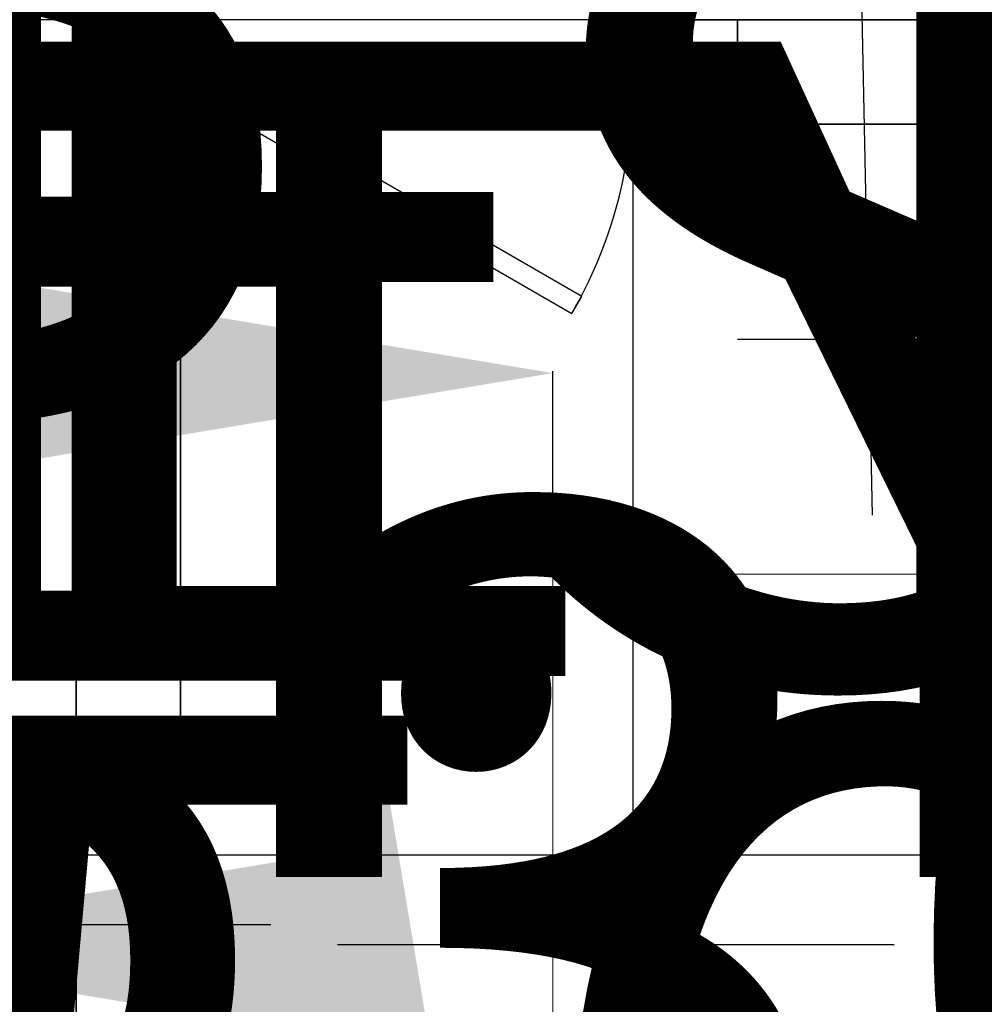
# Model space of a CAD drawing. Units: inches. Extents: x -307 to 2141, y -58 to 895.
# Tile 15 of 28: x 749 to 833, y 396 to 481. Entities that reach past the tile are written whole.
import ezdxf

# ---------------------------------------------------------------- set-up
doc = ezdxf.new("R2010")
doc.units = ezdxf.units.IN
doc.header["$MEASUREMENT"] = 0
for name, color, linetype, lineweight in [('A-ANNO-DIMS', 2, 'Continuous', 18), ('A-DOOR', 3, 'Continuous', 25), ('A-FURN', 8, 'Continuous', 18), ('A-WALL', 7, 'Continuous', 35)]:
    doc.layers.add(name, color=color, linetype=linetype, lineweight=lineweight)
doc.styles.get("Standard").update_dxf_attribs({"font": 'arial.ttf'})
doc.dimstyles.get("Standard").update_dxf_attribs({"dimtxt": 72, "dimasz": 48, "dimexe": 0.18, "dimexo": 0.0625, "dimgap": 0.09, "dimtad": 0, "dimtih": 1, "dimtoh": 1, "dimdec": 0, "dimrnd": 48, "dimzin": 0, "dimdsep": 46, "dimlunit": 3, "dimtxsty": 'Standard', "dimcen": 0.09, "dimadec": 0, "dimazin": 0, "dimtfac": 1, "dimtdec": 0, "dimtofl": 0, "dimtmove": 0, "dimatfit": 3, "dimfxl": 1, "dimtolj": 1, "dimtzin": 0, "dimarcsym": 0})

# ---------------------------------------------------------------- blocks, each defined once
blk = doc.blocks.new('*U5')
for p, q in [((0, 0), (0, -6)), ((-40, 0), (-40, -6))]:
    blk.add_line(p, q)
blk.add_lwpolyline([(0, 0), (-34.641, 20), (-35.516, 18.484), (-0.875, -1.516)], close=True)
blk.add_arc((0, 0), 40, 150, 180)
blk = doc.blocks.new('Bed - Queen')
for p, q in [((59.99999, 0), (59.99999, -80.00003)), ((59.99999, -80.00003), (0, -80.00003))]:
    blk.add_line(p, q)
blk = doc.blocks.new('*D28')
at = {"layer": 'A-ANNO-DIMS', "color": 0, "lineweight": -2, "transparency": 16777216}
for p, q in [((795.358, 433.55), (777.919, 433.55)), ((778.099, 385.55), (778.099, 366.073)), ((795.358, 318.073), (777.919, 318.073)), ((778.099, 318.073), (778.099, 270.073)), ((778.099, 270.073), (730.099, 270.073))]:
    blk.add_line(p, q, dxfattribs=at)
at = {"layer": 'A-ANNO-DIMS', "color": 0, "transparency": 16777216}
for points in [[(770.099, 385.55), (786.099, 385.55), (778.099, 433.55)], [(770.099, 366.073), (786.099, 366.073), (778.099, 318.073)]]:
    blk.add_solid(points, dxfattribs=at)
at = {"layer": 'Defpoints', "color": 0, "transparency": 16777216}
for p in [(795.421, 433.55), (778.099, 318.073), (795.421, 318.073)]:
    blk.add_point(p, dxfattribs=at)
at = {"layer": 'A-ANNO-DIMS', "color": 0, "transparency": 16777216, "insert": (534.416, 270.073), "char_height": 72, "attachment_point": 5}
blk.add_mtext('\\A1;BED 115', dxfattribs=at)
blk = doc.blocks.new('*D29')
at = {"layer": 'A-ANNO-DIMS', "color": 0, "lineweight": -2, "transparency": 16777216}
for p, q in [((747.421, 450.871), (699.421, 450.871)), ((795.421, 433.612), (795.421, 451.051)), ((882.028, 433.612), (882.028, 451.051)), ((930.028, 450.871), (978.028, 450.871))]:
    blk.add_line(p, q, dxfattribs=at)
at = {"layer": 'A-ANNO-DIMS', "color": 0, "transparency": 16777216}
for points in [[(747.421, 458.871), (747.421, 442.871), (795.421, 450.871)], [(930.028, 458.871), (930.028, 442.871), (882.028, 450.871)]]:
    blk.add_solid(points, dxfattribs=at)
at = {"layer": 'Defpoints', "color": 0, "transparency": 16777216}
for p in [(795.421, 450.871), (795.421, 433.55), (882.028, 433.55)]:
    blk.add_point(p, dxfattribs=at)
at = {"layer": 'A-ANNO-DIMS', "color": 0, "transparency": 16777216, "insert": (647.713, 450.871), "char_height": 72, "attachment_point": 5}
blk.add_mtext('\\A1;87', dxfattribs=at)
blk = doc.blocks.new('*D30')
at = {"layer": 'A-ANNO-DIMS', "color": 0, "lineweight": -2, "transparency": 16777216}
for p, q in [((570.736, 532.833), (570.736, 580.833)), ((570.736, 580.833), (618.736, 580.833)), ((565.398, 484.833), (570.916, 484.833)), ((565.398, 448.833), (570.916, 448.833)), ((570.736, 400.833), (570.736, 352.833))]:
    blk.add_line(p, q, dxfattribs=at)
at = {"layer": 'A-ANNO-DIMS', "color": 0, "transparency": 16777216}
for points in [[(562.736, 532.833), (578.736, 532.833), (570.736, 484.833)], [(562.736, 400.833), (578.736, 400.833), (570.736, 448.833)]]:
    blk.add_solid(points, dxfattribs=at)
at = {"layer": 'Defpoints', "color": 0, "transparency": 16777216}
for p in [(565.336, 484.833), (570.736, 484.833), (565.336, 448.833)]:
    blk.add_point(p, dxfattribs=at)
at = {"layer": 'A-ANNO-DIMS', "color": 0, "transparency": 16777216, "insert": (1030.174, 580.833), "char_height": 72, "attachment_point": 5}
blk.add_mtext('\\A1;WINDOW 36 TYP.', dxfattribs=at)
blk = doc.blocks.new('*D31')
at = {"layer": 'A-ANNO-DIMS', "color": 0, "lineweight": -2, "transparency": 16777216}
for p, q in [((556.336, 448.771), (556.336, 443.253)), ((565.336, 448.771), (565.336, 443.253)), ((508.336, 443.433), (460.336, 443.433)), ((613.336, 443.433), (661.336, 443.433))]:
    blk.add_line(p, q, dxfattribs=at)
at = {"layer": 'A-ANNO-DIMS', "color": 0, "transparency": 16777216}
for points in [[(508.336, 451.433), (508.336, 435.433), (556.336, 443.433)], [(613.336, 451.433), (613.336, 435.433), (565.336, 443.433)]]:
    blk.add_solid(points, dxfattribs=at)
at = {"layer": 'Defpoints', "color": 0, "transparency": 16777216}
for p in [(556.336, 448.833), (565.336, 448.833), (565.336, 443.433)]:
    blk.add_point(p, dxfattribs=at)
at = {"layer": 'A-ANNO-DIMS', "color": 0, "transparency": 16777216, "insert": (808.692, 443.433), "char_height": 72, "attachment_point": 5}
blk.add_mtext('\\A1;9 TYP.', dxfattribs=at)
blk = doc.blocks.new('*D35')
at = {"layer": 'A-ANNO-DIMS', "color": 0, "lineweight": -2, "transparency": 16777216}
for p, q in [((859.336, 453.769), (811.336, 453.769)), ((907.336, 443.029), (907.336, 453.949)), ((916.336, 443.029), (916.336, 453.949)), ((964.336, 453.769), (1012.336, 453.769))]:
    blk.add_line(p, q, dxfattribs=at)
at = {"layer": 'A-ANNO-DIMS', "color": 0, "transparency": 16777216}
for points in [[(859.336, 461.769), (859.336, 445.769), (907.336, 453.769)], [(964.336, 461.769), (964.336, 445.769), (916.336, 453.769)]]:
    blk.add_solid(points, dxfattribs=at)
at = {"layer": 'Defpoints', "color": 0, "transparency": 16777216}
for p in [(907.336, 453.769), (907.336, 442.967), (916.336, 442.967)]:
    blk.add_point(p, dxfattribs=at)
at = {"layer": 'A-ANNO-DIMS', "color": 0, "transparency": 16777216, "insert": (663.98, 453.769), "char_height": 72, "attachment_point": 5}
blk.add_mtext('\\A1;9 TYP.', dxfattribs=at)
blk = doc.blocks.new('*D36')
at = {"layer": 'A-ANNO-DIMS', "color": 0, "lineweight": -2, "transparency": 16777216}
for p, q in [((871.707, 562.404), (871.761, 610.404)), ((876.548, 514.399), (871.474, 514.405)), ((876.511, 481.353), (871.437, 481.358)), ((871.563, 433.358), (871.509, 385.358)), ((871.509, 385.358), (823.509, 385.358))]:
    blk.add_line(p, q, dxfattribs=at)
at = {"layer": 'A-ANNO-DIMS', "color": 0, "transparency": 16777216}
for points in [[(863.707, 562.413), (879.707, 562.395), (871.654, 514.404)], [(863.563, 433.367), (879.563, 433.349), (871.617, 481.358)]]:
    blk.add_solid(points, dxfattribs=at)
at = {"layer": 'Defpoints', "color": 0, "transparency": 16777216}
for p in [(876.611, 514.399), (871.617, 481.358), (876.574, 481.353)]:
    blk.add_point(p, dxfattribs=at)
at = {"layer": 'A-ANNO-DIMS', "color": 0, "transparency": 16777216, "insert": (548.95, 385.358), "char_height": 72, "attachment_point": 5}
blk.add_mtext('\\A1;WC 33 TYP.', dxfattribs=at)
blk = doc.blocks.new('*D37')
at = {"layer": 'A-ANNO-DIMS', "color": 0, "lineweight": -2, "transparency": 16777216}
for p, q in [((876.611, 514.461), (876.616, 519.536)), ((828.616, 519.409), (780.616, 519.463)), ((897.611, 514.438), (897.616, 519.512)), ((945.616, 519.279), (993.616, 519.225))]:
    blk.add_line(p, q, dxfattribs=at)
at = {"layer": 'A-ANNO-DIMS', "color": 0, "transparency": 16777216}
for points in [[(828.625, 527.409), (828.607, 511.409), (876.616, 519.356)], [(945.625, 527.279), (945.607, 511.279), (897.616, 519.332)]]:
    blk.add_solid(points, dxfattribs=at)
at = {"layer": 'Defpoints', "color": 0, "transparency": 16777216}
for p in [(876.616, 519.356), (876.611, 514.399), (897.611, 514.375)]:
    blk.add_point(p, dxfattribs=at)
at = {"layer": 'A-ANNO-DIMS', "color": 0, "transparency": 16777216, "insert": (604.676, 519.463), "char_height": 72, "attachment_point": 5}
blk.add_mtext('\\A1;21 TYP.', dxfattribs=at)
blk = doc.blocks.new('*D42')
at = {"layer": 'A-ANNO-DIMS', "color": 0, "lineweight": -2, "transparency": 16777216}
for p, q in [((880.259, 543.859), (928.248, 544.868)), ((822.302, 541.203), (822.268, 542.82)), ((832.299, 541.413), (832.265, 543.03)), ((774.282, 541.631), (726.293, 540.622))]:
    blk.add_line(p, q, dxfattribs=at)
at = {"layer": 'A-ANNO-DIMS', "color": 0, "transparency": 16777216}
for points in [[(880.09, 551.857), (880.427, 535.861), (832.269, 542.85)], [(774.114, 549.629), (774.45, 533.633), (822.271, 542.64)]]:
    blk.add_solid(points, dxfattribs=at)
at = {"layer": 'Defpoints', "color": 0, "transparency": 16777216}
for p in [(832.269, 542.85), (822.303, 541.14), (832.301, 541.35)]:
    blk.add_point(p, dxfattribs=at)
at = {"layer": 'A-ANNO-DIMS', "color": 0, "transparency": 16777216, "insert": (1192.886, 544.868), "char_height": 72, "attachment_point": 5}
blk.add_mtext('\\A1;FAUCET 10', dxfattribs=at)
blk = doc.blocks.new('*D43')
at = {"layer": 'A-ANNO-DIMS', "color": 0, "lineweight": -2, "transparency": 16777216}
for p, q in [((818.785, 637.088), (770.785, 637.088)), ((819.794, 589.098), (818.785, 637.088)), ((822.24, 541.139), (820.623, 541.105)), ((822.377, 534.64), (820.76, 534.606)), ((821.949, 486.621), (822.958, 438.631))]:
    blk.add_line(p, q, dxfattribs=at)
at = {"layer": 'A-ANNO-DIMS', "color": 0, "transparency": 16777216}
for points in [[(827.792, 589.266), (811.796, 588.93), (820.803, 541.109)], [(829.947, 486.789), (813.951, 486.453), (820.94, 534.61)]]:
    blk.add_solid(points, dxfattribs=at)
at = {"layer": 'Defpoints', "color": 0, "transparency": 16777216}
for p in [(820.803, 541.109), (822.303, 541.14), (822.44, 534.642)]:
    blk.add_point(p, dxfattribs=at)
at = {"layer": 'A-ANNO-DIMS', "color": 0, "transparency": 16777216, "insert": (747.391, 637.088), "char_height": 72, "attachment_point": 5}
blk.add_mtext('\\A1;7', dxfattribs=at)
blk = doc.blocks.new('*D44')
at = {"layer": 'A-ANNO-DIMS', "color": 0, "lineweight": -2, "transparency": 16777216}
for p, q in [((839.872, 521.223), (839.952, 517.424)), ((815.327, 520.707), (815.406, 516.907)), ((887.938, 518.613), (935.927, 519.622)), ((767.413, 516.078), (719.424, 515.069))]:
    blk.add_line(p, q, dxfattribs=at)
at = {"layer": 'A-ANNO-DIMS', "color": 0, "transparency": 16777216}
for points in [[(887.769, 526.611), (888.106, 510.614), (839.948, 517.604)], [(767.245, 524.076), (767.581, 508.08), (815.403, 517.087)]]:
    blk.add_solid(points, dxfattribs=at)
at = {"layer": 'Defpoints', "color": 0, "transparency": 16777216}
for p in [(839.871, 521.285), (815.325, 520.769), (839.948, 517.604)]:
    blk.add_point(p, dxfattribs=at)
at = {"layer": 'A-ANNO-DIMS', "color": 0, "transparency": 16777216, "insert": (1151.157, 519.622), "char_height": 72, "attachment_point": 5}
blk.add_mtext('\\A1;BASIN 25', dxfattribs=at)
blk = doc.blocks.new('*D45')
at = {"layer": 'A-ANNO-DIMS', "color": 0, "lineweight": -2, "transparency": 16777216}
for p, q in [((841.111, 637.474), (793.111, 637.474)), ((842.12, 589.484), (841.111, 637.474)), ((839.51, 541.419), (843.309, 541.499)), ((839.933, 521.287), (843.732, 521.367)), ((844.562, 473.373), (845.571, 425.384))]:
    blk.add_line(p, q, dxfattribs=at)
at = {"layer": 'A-ANNO-DIMS', "color": 0, "transparency": 16777216}
for points in [[(850.118, 589.652), (834.122, 589.316), (843.129, 541.495)], [(852.56, 473.542), (836.563, 473.205), (843.553, 521.363)]]:
    blk.add_solid(points, dxfattribs=at)
at = {"layer": 'Defpoints', "color": 0, "transparency": 16777216}
for p in [(839.447, 541.417), (843.129, 541.495), (839.871, 521.285)]:
    blk.add_point(p, dxfattribs=at)
at = {"layer": 'A-ANNO-DIMS', "color": 0, "transparency": 16777216, "insert": (740.961, 637.474), "char_height": 72, "attachment_point": 5}
blk.add_mtext('\\A1;20', dxfattribs=at)
blk = doc.blocks.new('*D46')
at = {"layer": 'A-ANNO-DIMS', "color": 0, "lineweight": -2, "transparency": 16777216}
for p, q in [((801.413, 645.783), (801.413, 642.516)), ((822.413, 645.783), (822.413, 642.516)), ((753.413, 642.696), (705.413, 642.696)), ((870.413, 642.696), (918.413, 642.696))]:
    blk.add_line(p, q, dxfattribs=at)
at = {"layer": 'A-ANNO-DIMS', "color": 0, "transparency": 16777216}
for points in [[(753.413, 650.696), (753.413, 634.696), (801.413, 642.696)], [(870.413, 650.696), (870.413, 634.696), (822.413, 642.696)]]:
    blk.add_solid(points, dxfattribs=at)
at = {"layer": 'Defpoints', "color": 0, "transparency": 16777216}
for p in [(801.413, 645.846), (822.413, 645.846), (822.413, 642.696)]:
    blk.add_point(p, dxfattribs=at)
at = {"layer": 'A-ANNO-DIMS', "color": 0, "transparency": 16777216, "insert": (1282.702, 642.696), "char_height": 72, "attachment_point": 5}
blk.add_mtext('\\A1;DESK CHAIR 21', dxfattribs=at)
blk = doc.blocks.new('*D52')
at = {"layer": 'A-ANNO-DIMS', "color": 0, "lineweight": -2, "transparency": 16777216}
for p, q in [((660.208, 554.249), (660.208, 602.249)), ((673.796, 506.249), (660.028, 506.249)), ((673.796, 415.249), (660.028, 415.249)), ((660.208, 367.249), (660.208, 319.249))]:
    blk.add_line(p, q, dxfattribs=at)
at = {"layer": 'A-ANNO-DIMS', "color": 0, "transparency": 16777216}
for points in [[(652.208, 554.249), (668.208, 554.249), (660.208, 506.249)], [(652.208, 367.249), (668.208, 367.249), (660.208, 415.249)]]:
    blk.add_solid(points, dxfattribs=at)
at = {"layer": 'Defpoints', "color": 0, "transparency": 16777216}
for p in [(673.858, 506.249), (660.208, 415.249), (673.858, 415.249)]:
    blk.add_point(p, dxfattribs=at)
at = {"layer": 'A-ANNO-DIMS', "color": 0, "transparency": 16777216, "insert": (660.208, 460.749), "char_height": 72, "attachment_point": 5}
blk.add_mtext('\\A1;DINING SET 91', dxfattribs=at)
blk = doc.blocks.new('*D53')
at = {"layer": 'A-ANNO-DIMS', "color": 0, "lineweight": -2, "transparency": 16777216}
for p, q in [((673.858, 415.186), (673.858, 401.419)), ((728.858, 415.186), (728.858, 401.419)), ((625.858, 401.599), (577.858, 401.599)), ((776.858, 401.599), (824.858, 401.599))]:
    blk.add_line(p, q, dxfattribs=at)
at = {"layer": 'A-ANNO-DIMS', "color": 0, "transparency": 16777216}
for points in [[(625.858, 409.599), (625.858, 393.599), (673.858, 401.599)], [(776.858, 409.599), (776.858, 393.599), (728.858, 401.599)]]:
    blk.add_solid(points, dxfattribs=at)
at = {"layer": 'Defpoints', "color": 0, "transparency": 16777216}
for p in [(673.858, 415.249), (728.858, 415.249), (728.858, 401.599)]:
    blk.add_point(p, dxfattribs=at)
at = {"layer": 'A-ANNO-DIMS', "color": 0, "transparency": 16777216, "insert": (876.787, 401.599), "char_height": 72, "attachment_point": 5}
blk.add_mtext('\\A1;55', dxfattribs=at)
blk = doc.blocks.new('*D54')
at = {"layer": 'A-ANNO-DIMS', "color": 0, "lineweight": -2, "transparency": 16777216}
for p, q in [((605.336, 412.349), (605.336, 460.349)), ((605.336, 460.349), (653.336, 460.349)), ((596.398, 364.349), (605.516, 364.349)), ((596.398, 304.349), (605.516, 304.349)), ((605.336, 256.349), (605.336, 208.349))]:
    blk.add_line(p, q, dxfattribs=at)
at = {"layer": 'A-ANNO-DIMS', "color": 0, "transparency": 16777216}
for points in [[(597.336, 412.349), (613.336, 412.349), (605.336, 364.349)], [(597.336, 256.349), (613.336, 256.349), (605.336, 304.349)]]:
    blk.add_solid(points, dxfattribs=at)
at = {"layer": 'Defpoints', "color": 0, "transparency": 16777216}
for p in [(596.336, 364.349), (605.336, 364.349), (596.336, 304.349)]:
    blk.add_point(p, dxfattribs=at)
at = {"layer": 'A-ANNO-DIMS', "color": 0, "transparency": 16777216, "insert": (854.004, 460.349), "char_height": 72, "attachment_point": 5}
blk.add_mtext('\\A1;DESK 60', dxfattribs=at)
blk = doc.blocks.new('*D60')
at = {"layer": 'A-ANNO-DIMS', "color": 0, "lineweight": -2, "transparency": 16777216}
for p, q in [((659.857, 294.946), (659.857, 342.946)), ((659.857, 342.946), (707.857, 342.946)), ((663.339, 246.946), (659.677, 246.946)), ((663.339, 223.315), (659.677, 223.315)), ((659.857, 175.315), (659.857, 127.315))]:
    blk.add_line(p, q, dxfattribs=at)
at = {"layer": 'A-ANNO-DIMS', "color": 0, "transparency": 16777216}
for points in [[(651.857, 294.946), (667.857, 294.946), (659.857, 246.946)], [(651.857, 175.315), (667.857, 175.315), (659.857, 223.315)]]:
    blk.add_solid(points, dxfattribs=at)
at = {"layer": 'Defpoints', "color": 0, "transparency": 16777216}
for p in [(659.857, 246.946), (663.402, 246.946), (663.402, 223.315)]:
    blk.add_point(p, dxfattribs=at)
at = {"layer": 'A-ANNO-DIMS', "color": 0, "transparency": 16777216, "insert": (933.573, 342.946), "char_height": 72, "attachment_point": 5}
blk.add_mtext('\\A1;TABLE 24', dxfattribs=at)
blk = doc.blocks.new('*D63')
at = {"layer": 'A-ANNO-DIMS', "color": 0, "lineweight": -2, "transparency": 16777216}
for p, q in [((916.398, 691.341), (947.72, 691.341)), ((947.54, 643.341), (947.54, 416.192)), ((947.54, 115.341), (947.54, 342.49)), ((704.684, 67.341), (947.72, 67.341))]:
    blk.add_line(p, q, dxfattribs=at)
at = {"layer": 'A-ANNO-DIMS', "color": 0, "transparency": 16777216}
for points in [[(939.54, 643.341), (955.54, 643.341), (947.54, 691.341)], [(939.54, 115.341), (955.54, 115.341), (947.54, 67.341)]]:
    blk.add_solid(points, dxfattribs=at)
at = {"layer": 'Defpoints', "color": 0, "transparency": 16777216}
for p in [(916.336, 691.341), (704.621, 67.341), (947.54, 67.341)]:
    blk.add_point(p, dxfattribs=at)
at = {"layer": 'A-ANNO-DIMS', "color": 0, "transparency": 16777216, "insert": (947.54, 379.341), "char_height": 72, "attachment_point": 5}
blk.add_mtext('\\A1;624', dxfattribs=at)
blk = doc.blocks.new('*D68')
at = {"layer": 'A-ANNO-DIMS', "color": 0, "lineweight": -2, "transparency": 16777216}
for p, q in [((525.132, 586.341), (525.132, 634.341)), ((525.132, 634.341), (573.132, 634.341)), ((565.273, 538.341), (524.952, 538.341)), ((556.273, 484.833), (524.952, 484.833)), ((525.132, 436.833), (525.132, 388.833))]:
    blk.add_line(p, q, dxfattribs=at)
at = {"layer": 'A-ANNO-DIMS', "color": 0, "transparency": 16777216}
for points in [[(517.132, 586.341), (533.132, 586.341), (525.132, 538.341)], [(517.132, 436.833), (533.132, 436.833), (525.132, 484.833)]]:
    blk.add_solid(points, dxfattribs=at)
at = {"layer": 'Defpoints', "color": 0, "transparency": 16777216}
for p in [(525.132, 538.341), (565.336, 538.341), (556.336, 484.833)]:
    blk.add_point(p, dxfattribs=at)
at = {"layer": 'A-ANNO-DIMS', "color": 0, "transparency": 16777216, "insert": (687.754, 634.341), "char_height": 72, "attachment_point": 5}
blk.add_mtext('\\A1;53.51', dxfattribs=at)
blk = doc.blocks.new('*D82')
at = {"layer": 'A-ANNO-DIMS', "color": 0, "lineweight": -2, "transparency": 16777216}
for p, q in [((525.132, 565.341), (525.132, 613.341)), ((525.132, 613.341), (573.132, 613.341)), ((802.273, 517.341), (524.952, 517.341)), ((802.273, 481.341), (524.952, 481.341)), ((525.132, 433.341), (525.132, 385.341))]:
    blk.add_line(p, q, dxfattribs=at)
at = {"layer": 'A-ANNO-DIMS', "color": 0, "transparency": 16777216}
for points in [[(517.132, 565.341), (533.132, 565.341), (525.132, 517.341)], [(517.132, 433.341), (533.132, 433.341), (525.132, 481.341)]]:
    blk.add_solid(points, dxfattribs=at)
at = {"layer": 'Defpoints', "color": 0, "transparency": 16777216}
for p in [(525.132, 517.341), (802.336, 517.341), (802.336, 481.341)]:
    blk.add_point(p, dxfattribs=at)
at = {"layer": 'A-ANNO-DIMS', "color": 0, "transparency": 16777216, "insert": (624.742, 613.341), "char_height": 72, "attachment_point": 5}
blk.add_mtext('\\A1;36', dxfattribs=at)
blk = doc.blocks.new('*D83')
at = {"layer": 'A-ANNO-DIMS', "color": 0, "lineweight": -2, "transparency": 16777216}
for p, q in [((947.54, 538.903), (947.54, 586.903)), ((916.398, 490.903), (947.72, 490.903)), ((907.398, 481.341), (947.72, 481.341)), ((947.54, 433.341), (947.54, 385.341)), ((947.54, 385.341), (899.54, 385.341))]:
    blk.add_line(p, q, dxfattribs=at)
at = {"layer": 'A-ANNO-DIMS', "color": 0, "transparency": 16777216}
for points in [[(939.54, 538.903), (955.54, 538.903), (947.54, 490.903)], [(939.54, 433.341), (955.54, 433.341), (947.54, 481.341)]]:
    blk.add_solid(points, dxfattribs=at)
at = {"layer": 'Defpoints', "color": 0, "transparency": 16777216}
for p in [(916.336, 490.903), (907.336, 481.341), (947.54, 481.341)]:
    blk.add_point(p, dxfattribs=at)
at = {"layer": 'A-ANNO-DIMS', "color": 0, "transparency": 16777216, "insert": (777.968, 385.341), "char_height": 72, "attachment_point": 5}
blk.add_mtext('\\A1;9.563', dxfattribs=at)
blk = doc.blocks.new('*D84')
at = {"layer": 'A-ANNO-DIMS', "color": 0, "lineweight": -2, "transparency": 16777216}
for p, q in [((763.336, 472.278), (763.336, 35.957)), ((907.336, 472.278), (907.336, 35.957)), ((811.336, 36.137), (859.336, 36.137)), ((907.336, 36.137), (955.336, 36.137))]:
    blk.add_line(p, q, dxfattribs=at)
at = {"layer": 'A-ANNO-DIMS', "color": 0, "transparency": 16777216}
for points in [[(811.336, 44.137), (811.336, 28.137), (763.336, 36.137)], [(859.336, 44.137), (859.336, 28.137), (907.336, 36.137)]]:
    blk.add_solid(points, dxfattribs=at)
at = {"layer": 'Defpoints', "color": 0, "transparency": 16777216}
for p in [(763.336, 472.341), (907.336, 472.341), (907.336, 36.137)]:
    blk.add_point(p, dxfattribs=at)
at = {"layer": 'A-ANNO-DIMS', "color": 0, "transparency": 16777216, "insert": (1031.429, 36.137), "char_height": 72, "attachment_point": 5}
blk.add_mtext('\\A1;144', dxfattribs=at)
blk = doc.blocks.new('*D88')
at = {"layer": 'A-ANNO-DIMS', "color": 0, "lineweight": -2, "transparency": 16777216}
for p, q in [((517.33584, 722.544828), (469.33584, 722.544828)), ((565.33584, 295.403328), (565.33584, 722.724828)), ((754.33584, 271.403328), (754.33584, 722.724828)), ((802.33584, 722.544828), (850.33584, 722.544828))]:
    blk.add_line(p, q, dxfattribs=at)
at = {"layer": 'A-ANNO-DIMS', "color": 0, "transparency": 16777216}
for points in [[(517.33584, 730.544828), (517.33584, 714.544828), (565.33584, 722.544828)], [(802.33584, 730.544828), (802.33584, 714.544828), (754.33584, 722.544828)]]:
    blk.add_solid(points, dxfattribs=at)
at = {"layer": 'Defpoints', "color": 0, "transparency": 16777216}
for p in [(754.33584, 722.544828), (565.33584, 295.340828), (754.33584, 271.340828)]:
    blk.add_point(p, dxfattribs=at)
at = {"layer": 'A-ANNO-DIMS', "color": 0, "transparency": 16777216, "insert": (659.83584, 722.544828), "char_height": 72, "attachment_point": 5}
blk.add_mtext('\\A1;189', dxfattribs=at)
blk = doc.blocks.new('*D95')
at = {"layer": 'A-ANNO-DIMS', "color": 0, "lineweight": -2, "transparency": 16777216}
for p, q in [((947.54, 577.341), (947.54, 625.341)), ((947.54, 625.341), (995.54, 625.341)), ((629.898, 529.341), (947.72, 529.341)), ((629.898, 502.663), (947.72, 502.663)), ((947.54, 454.663), (947.54, 406.663))]:
    blk.add_line(p, q, dxfattribs=at)
at = {"layer": 'A-ANNO-DIMS', "color": 0, "transparency": 16777216}
for points in [[(939.54, 577.341), (955.54, 577.341), (947.54, 529.341)], [(939.54, 454.663), (955.54, 454.663), (947.54, 502.663)]]:
    blk.add_solid(points, dxfattribs=at)
at = {"layer": 'Defpoints', "color": 0, "transparency": 16777216}
for p in [(629.836, 529.341), (947.54, 529.341), (629.836, 502.663)]:
    blk.add_point(p, dxfattribs=at)
at = {"layer": 'A-ANNO-DIMS', "color": 0, "transparency": 16777216, "insert": (1117.799, 625.341), "char_height": 72, "attachment_point": 5}
blk.add_mtext('\\A1;26.68', dxfattribs=at)
blk = doc.blocks.new('*D97')
at = {"layer": 'A-ANNO-DIMS', "color": 0, "lineweight": -2, "transparency": 16777216}
for p, q in [((947.54, 637.341), (947.54, 685.341)), ((947.54, 685.341), (995.54, 685.341)), ((685.398, 589.341), (947.72, 589.341)), ((685.398, 538.341), (947.72, 538.341)), ((947.54, 490.341), (947.54, 442.341))]:
    blk.add_line(p, q, dxfattribs=at)
at = {"layer": 'A-ANNO-DIMS', "color": 0, "transparency": 16777216}
for points in [[(939.54, 637.341), (955.54, 637.341), (947.54, 589.341)], [(939.54, 490.341), (955.54, 490.341), (947.54, 538.341)]]:
    blk.add_solid(points, dxfattribs=at)
at = {"layer": 'Defpoints', "color": 0, "transparency": 16777216}
for p in [(685.336, 589.341), (947.54, 589.341), (685.336, 538.341)]:
    blk.add_point(p, dxfattribs=at)
at = {"layer": 'A-ANNO-DIMS', "color": 0, "transparency": 16777216, "insert": (1040.249, 685.341), "char_height": 72, "attachment_point": 5}
blk.add_mtext('\\A1;51', dxfattribs=at)
blk = doc.blocks.new('*D98')
at = {"layer": 'A-ANNO-DIMS', "color": 0, "lineweight": -2, "transparency": 16777216}
for p, q in [((525.132, 637.341), (525.132, 685.341)), ((525.132, 685.341), (573.132, 685.341)), ((787.273, 589.341), (524.952, 589.341)), ((787.273, 550.341), (524.952, 550.341)), ((525.132, 502.341), (525.132, 454.341))]:
    blk.add_line(p, q, dxfattribs=at)
at = {"layer": 'A-ANNO-DIMS', "color": 0, "transparency": 16777216}
for points in [[(517.132, 637.341), (533.132, 637.341), (525.132, 589.341)], [(517.132, 502.341), (533.132, 502.341), (525.132, 550.341)]]:
    blk.add_solid(points, dxfattribs=at)
at = {"layer": 'Defpoints', "color": 0, "transparency": 16777216}
for p in [(525.132, 589.341), (787.336, 589.341), (787.336, 550.341)]:
    blk.add_point(p, dxfattribs=at)
at = {"layer": 'A-ANNO-DIMS', "color": 0, "transparency": 16777216, "insert": (624.84, 685.341), "char_height": 72, "attachment_point": 5}
blk.add_mtext('\\A1;39', dxfattribs=at)
blk = doc.blocks.new('*D99')
at = {"layer": 'A-ANNO-DIMS', "color": 0, "lineweight": -2, "transparency": 16777216}
for p, q in [((763.336, 481.278), (763.336, 35.957)), ((802.336, 481.278), (802.336, 35.957)), ((715.336, 36.137), (667.336, 36.137)), ((850.336, 36.137), (898.336, 36.137))]:
    blk.add_line(p, q, dxfattribs=at)
at = {"layer": 'A-ANNO-DIMS', "color": 0, "transparency": 16777216}
for points in [[(715.336, 44.137), (715.336, 28.137), (763.336, 36.137)], [(850.336, 44.137), (850.336, 28.137), (802.336, 36.137)]]:
    blk.add_solid(points, dxfattribs=at)
at = {"layer": 'Defpoints', "color": 0, "transparency": 16777216}
for p in [(763.336, 481.341), (802.336, 481.341), (802.336, 36.137)]:
    blk.add_point(p, dxfattribs=at)
at = {"layer": 'A-ANNO-DIMS', "color": 0, "transparency": 16777216, "insert": (950.044, 36.137), "char_height": 72, "attachment_point": 5}
blk.add_mtext('\\A1;39', dxfattribs=at)
blk = doc.blocks.new('*D100')
at = {"layer": 'A-ANNO-DIMS', "color": 0, "lineweight": -2, "transparency": 16777216}
for p, q in [((589.339, 409.278), (589.339, 35.957)), ((625.336, 409.278), (625.336, 35.957)), ((541.339, 36.137), (493.339, 36.137)), ((673.336, 36.137), (721.336, 36.137))]:
    blk.add_line(p, q, dxfattribs=at)
at = {"layer": 'A-ANNO-DIMS', "color": 0, "transparency": 16777216}
for points in [[(541.339, 44.137), (541.339, 28.137), (589.339, 36.137)], [(673.336, 44.137), (673.336, 28.137), (625.336, 36.137)]]:
    blk.add_solid(points, dxfattribs=at)
at = {"layer": 'Defpoints', "color": 0, "transparency": 16777216}
for p in [(589.339, 409.341), (625.336, 409.341), (625.336, 36.137)]:
    blk.add_point(p, dxfattribs=at)
at = {"layer": 'A-ANNO-DIMS', "color": 0, "transparency": 16777216, "insert": (772.946, 36.137), "char_height": 72, "attachment_point": 5}
blk.add_mtext('\\A1;36', dxfattribs=at)
blk = doc.blocks.new('*D107')
at = {"layer": 'A-ANNO-DIMS', "color": 0, "lineweight": -2, "transparency": 16777216}
for p, q in [((517.336, 722.545), (469.336, 722.545)), ((565.336, 409.403), (565.336, 722.725)), ((589.339, 409.403), (589.339, 722.725)), ((637.339, 722.545), (685.339, 722.545))]:
    blk.add_line(p, q, dxfattribs=at)
at = {"layer": 'A-ANNO-DIMS', "color": 0, "transparency": 16777216}
for points in [[(517.336, 730.545), (517.336, 714.545), (565.336, 722.545)], [(637.339, 730.545), (637.339, 714.545), (589.339, 722.545)]]:
    blk.add_solid(points, dxfattribs=at)
at = {"layer": 'Defpoints', "color": 0, "transparency": 16777216}
for p in [(589.339, 722.545), (565.336, 409.341), (589.339, 409.341)]:
    blk.add_point(p, dxfattribs=at)
at = {"layer": 'A-ANNO-DIMS', "color": 0, "transparency": 16777216, "insert": (835.495, 722.545), "char_height": 72, "attachment_point": 5}
blk.add_mtext('\\A1;24.003', dxfattribs=at)
blk = doc.blocks.new('*D108')
at = {"layer": 'A-ANNO-DIMS', "color": 0, "lineweight": -2, "transparency": 16777216}
for p, q in [((947.54, 550.663), (947.54, 598.663)), ((589.402, 502.663), (947.72, 502.663)), ((589.402, 409.341), (947.72, 409.341)), ((947.54, 361.341), (947.54, 313.341))]:
    blk.add_line(p, q, dxfattribs=at)
at = {"layer": 'A-ANNO-DIMS', "color": 0, "transparency": 16777216}
for points in [[(939.54, 550.663), (955.54, 550.663), (947.54, 502.663)], [(939.54, 361.341), (955.54, 361.341), (947.54, 409.341)]]:
    blk.add_solid(points, dxfattribs=at)
at = {"layer": 'Defpoints', "color": 0, "transparency": 16777216}
for p in [(589.339, 502.663), (947.54, 502.663), (589.339, 409.341)]:
    blk.add_point(p, dxfattribs=at)
at = {"layer": 'A-ANNO-DIMS', "color": 0, "transparency": 16777216, "insert": (947.54, 456.002), "char_height": 72, "attachment_point": 5}
blk.add_mtext('\\A1;93.32', dxfattribs=at)
blk = doc.blocks.new('*D109')
at = {"layer": 'A-ANNO-DIMS', "color": 0, "lineweight": -2, "transparency": 16777216}
for p, q in [((723.132, 355.341), (723.132, 403.341)), ((723.132, 403.341), (771.132, 403.341)), ((754.273, 307.341), (722.952, 307.341)), ((754.273, 271.341), (722.952, 271.341)), ((723.132, 223.341), (723.132, 175.341))]:
    blk.add_line(p, q, dxfattribs=at)
at = {"layer": 'A-ANNO-DIMS', "color": 0, "transparency": 16777216}
for points in [[(715.132, 355.341), (731.132, 355.341), (723.132, 307.341)], [(715.132, 223.341), (731.132, 223.341), (723.132, 271.341)]]:
    blk.add_solid(points, dxfattribs=at)
at = {"layer": 'Defpoints', "color": 0, "transparency": 16777216}
for p in [(723.132, 307.341), (754.336, 307.341), (754.336, 271.341)]:
    blk.add_point(p, dxfattribs=at)
at = {"layer": 'A-ANNO-DIMS', "color": 0, "transparency": 16777216, "insert": (822.742, 403.341), "char_height": 72, "attachment_point": 5}
blk.add_mtext('\\A1;36', dxfattribs=at)

msp = doc.modelspace()

# ---------------------------------------------------------------- linework, layer by layer
at = {"layer": 'A-WALL'}
for p, q in [((754.3358, 307.3408), (754.3358, 481.3408)), ((754.3358, 307.3408), (754.3358, 481.3408)), ((763.3358, 481.3408), (754.3358, 481.3408)), ((763.3358, 307.3408), (763.3358, 481.3408)), ((763.3358, 307.3408), (763.3358, 481.3408)), ((907.3358, 481.3408), (802.3358, 481.3408)), ((802.3358, 472.3408), (802.3358, 481.3408)), ((907.3358, 481.3408), (802.3358, 481.3408)), ((811.3358, 472.3408), (811.3358, 481.3408)), ((763.3358, 472.3408), (754.3358, 472.3408)), ((907.3358, 472.3408), (802.3358, 472.3408))]:
    msp.add_line(p, q, dxfattribs=at)

# ---------------------------------------------------------------- block references
at = {"layer": 'A-DOOR', "xscale": 0.9741143444065041, "yscale": 0.9741143444065041, "zscale": 0.9741143444065041, "rotation": 179.9999999999999}
msp.add_blockref('*U5', (763.3358, 475.4961), dxfattribs=at)
at = {"layer": 'A-FURN', "xscale": 1.443457686913744, "yscale": 1.443457686913744, "zscale": 1.443457686913744, "rotation": 179.9999999999998}
msp.add_blockref('Bed - Queen', (882.0282, 318.073), dxfattribs=at)

# ---------------------------------------------------------------- dimensions: what is measured, and where the dimension line sits
at = {"layer": 'A-ANNO-DIMS'}
for base, p1, p2, text, picture, middle in [((822.4132, 642.696), (801.4132, 645.846), (822.4132, 645.846), 'DESK CHAIR <>', '*D46', (1282.7024, 642.696)), ((565.3358, 443.4333), (556.3358, 448.8333), (565.3358, 448.8333), '<> TYP.', '*D31', (808.6919, 443.4333))]:
    dim = msp.add_linear_dim(base=base, p1=p1, p2=p2, text=text, dimstyle='Standard', override={"dimdec": 0, "dimlfac": 1, "dimrnd": 0, "dimzin": 0, "dimdsep": 46, "dimlunit": 2}, dxfattribs=at)
    dim.commit()
    dim.dimension.update_dxf_attribs({"geometry": picture, "text_midpoint": middle})
for base, p1, p2, override, picture, middle in [((754.3358, 722.5448), (565.3358, 295.3408), (754.3358, 271.3408), {"dimdec": 0, "dimlfac": 1, "dimrnd": 0, "dimzin": 0, "dimdsep": 46, "dimlunit": 2}, '*D88', (659.8358, 722.5448)), ((589.339, 722.5448), (565.3358, 409.3408), (589.339, 409.3408), {"dimdec": 3, "dimlfac": 1, "dimrnd": 0, "dimzin": 0, "dimdsep": 46, "dimlunit": 2}, '*D107', (835.4945, 722.5448)), ((802.3358, 36.1368), (763.3358, 481.3408), (802.3358, 481.3408), {"dimdec": 0, "dimlfac": 1, "dimrnd": 0, "dimzin": 0, "dimdsep": 46, "dimlunit": 2}, '*D99', (950.0438, 36.1368)), ((907.3358, 36.1368), (763.3358, 472.3408), (907.3358, 472.3408), {"dimdec": 0, "dimlfac": 1, "dimrnd": 0, "dimzin": 0, "dimdsep": 46, "dimlunit": 2}, '*D84', (1031.4286, 36.1368)), ((728.8583, 401.5985), (673.8583, 415.2485), (728.8583, 415.2485), {"dimdec": 0, "dimlfac": 1, "dimrnd": 0, "dimzin": 0, "dimdsep": 46, "dimlunit": 2}, '*D53', (876.7874, 401.5985)), ((625.3358, 36.1368), (589.339, 409.3408), (625.3358, 409.3408), {"dimdec": 0, "dimlfac": 1, "dimrnd": 0, "dimzin": 0, "dimdsep": 46, "dimlunit": 2}, '*D100', (772.9456, 36.1368))]:
    dim = msp.add_linear_dim(base=base, p1=p1, p2=p2, dimstyle='Standard', override=override, dxfattribs=at)
    dim.commit()
    dim.dimension.update_dxf_attribs({"geometry": picture, "text_midpoint": middle})
for base, p1, p2, angle, text, picture, middle in [((570.7358, 484.8333), (565.3358, 448.8333), (565.3358, 484.8333), 90, 'WINDOW <> TYP.', '*D30', (1030.1737, 580.8333)), ((832.2692, 542.8502), (822.3029, 541.1403), (832.3007, 541.3505), 1.204628, 'FAUCET <>', '*D42', (1192.8864, 544.8684)), ((660.2083, 415.2485), (673.8583, 506.2485), (673.8583, 415.2485), 270, 'DINING SET <>', '*D52', (660.2083, 460.7485)), ((876.6162, 519.3557), (897.6106, 514.3753), (876.6106, 514.3988), 179.935892, '<> TYP.', '*D37', (604.6763, 519.4631)), ((839.9481, 517.6035), (815.3253, 520.7692), (839.8707, 521.2853), 1.204628, 'BASIN <>', '*D44', (1151.1574, 519.6217)), ((871.6167, 481.3581), (876.6106, 514.3988), (876.5736, 481.3526), 269.935892, 'WC <> TYP.', '*D36', (548.95, 385.3582)), ((605.3358, 364.3488), (596.3358, 304.3488), (596.3358, 364.3488), 90, 'DESK <>', '*D54', (854.0043, 460.3488)), ((907.3358, 453.7692), (916.3358, 442.9669), (907.3358, 442.9669), 180, '<> TYP.', '*D35', (663.9798, 453.7692)), ((659.8571, 246.9465), (663.4018, 223.3153), (663.4018, 246.9465), 90, 'TABLE <>', '*D60', (933.5733, 342.9465)), ((778.0993, 318.073), (795.4208, 433.5496), (795.4208, 318.073), 270, 'BED <>', '*D28', (534.4158, 270.073))]:
    dim = msp.add_linear_dim(base=base, p1=p1, p2=p2, angle=angle, text=text, dimstyle='Standard', override={"dimdec": 0, "dimlfac": 1, "dimrnd": 0, "dimzin": 0, "dimdsep": 46, "dimlunit": 2}, dxfattribs=at)
    dim.commit()
    dim.dimension.update_dxf_attribs({"geometry": picture, "text_midpoint": middle})
for base, p1, p2, angle, override, picture, middle in [((525.1318, 589.3408), (787.3358, 550.3408), (787.3358, 589.3408), 90, {"dimdec": 0, "dimlfac": 1, "dimrnd": 0, "dimzin": 0, "dimdsep": 46, "dimlunit": 2}, '*D98', (624.8398, 685.3408)), ((947.5398, 589.3408), (685.3358, 538.3408), (685.3358, 589.3408), 90, {"dimdec": 0, "dimlfac": 1, "dimrnd": 0, "dimzin": 0, "dimdsep": 46, "dimlunit": 2}, '*D97', (1040.2492, 685.3408)), ((947.5398, 67.3408), (916.3358, 691.3408), (704.6211, 67.3408), 90, {"dimdec": 0, "dimlfac": 1, "dimrnd": 0, "dimzin": 0, "dimdsep": 46, "dimlunit": 2}, '*D63', (947.5398, 379.3408)), ((843.1292, 541.4949), (839.8707, 521.2853), (839.4474, 541.4175), 91.204628, {"dimdec": 0, "dimlfac": 1, "dimrnd": 0, "dimzin": 0, "dimdsep": 46, "dimlunit": 2}, '*D45', (740.961, 637.4737)), ((820.8033, 541.1087), (822.4396, 534.6416), (822.3029, 541.1403), 91.204628, {"dimdec": 0, "dimlfac": 1, "dimrnd": 0, "dimzin": 0, "dimdsep": 46, "dimlunit": 2}, '*D43', (747.3908, 637.0875)), ((525.1318, 538.3408), (556.3358, 484.8333), (565.3358, 538.3408), 90, {"dimdec": 2, "dimlfac": 1, "dimrnd": 0, "dimzin": 0, "dimdsep": 46, "dimlunit": 2}, '*D68', (687.7539, 634.3408)), ((947.5398, 529.3408), (629.8358, 502.6632), (629.8358, 529.3408), 90, {"dimdec": 2, "dimlfac": 1, "dimrnd": 0, "dimzin": 0, "dimdsep": 46, "dimlunit": 2}, '*D95', (1117.799, 625.3408)), ((525.1318, 517.3408), (802.3358, 481.3408), (802.3358, 517.3408), 90, {"dimdec": 0, "dimlfac": 1, "dimrnd": 0, "dimzin": 0, "dimdsep": 46, "dimlunit": 2}, '*D82', (624.7416, 613.3408)), ((947.5398, 502.6632), (589.339, 409.3408), (589.339, 502.6632), 90, {"dimdec": 2, "dimlfac": 1, "dimrnd": 0, "dimzin": 0, "dimdsep": 46, "dimlunit": 2}, '*D108', (947.5398, 456.002)), ((947.5398, 481.3408), (916.3358, 490.9034), (907.3358, 481.3408), 90, {"dimdec": 3, "dimlfac": 1, "dimrnd": 0, "dimzin": 0, "dimdsep": 46, "dimlunit": 2}, '*D83', (777.9683, 385.3408)), ((795.4208, 450.8711), (882.0282, 433.5496), (795.4208, 433.5496), 180, {"dimdec": 0, "dimlfac": 1, "dimrnd": 0, "dimzin": 0, "dimdsep": 46, "dimlunit": 2}, '*D29', (647.7128, 450.8711)), ((723.1318, 307.3408), (754.3358, 271.3408), (754.3358, 307.3408), 90, {"dimdec": 0, "dimlfac": 1, "dimrnd": 0, "dimzin": 0, "dimdsep": 46, "dimlunit": 2}, '*D109', (822.7416, 403.3408))]:
    dim = msp.add_linear_dim(base=base, p1=p1, p2=p2, angle=angle, dimstyle='Standard', override=override, dxfattribs=at)
    dim.commit()
    dim.dimension.update_dxf_attribs({"geometry": picture, "text_midpoint": middle})

doc.saveas('drawing.dxf')
